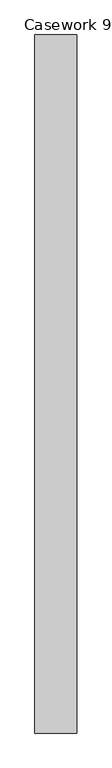
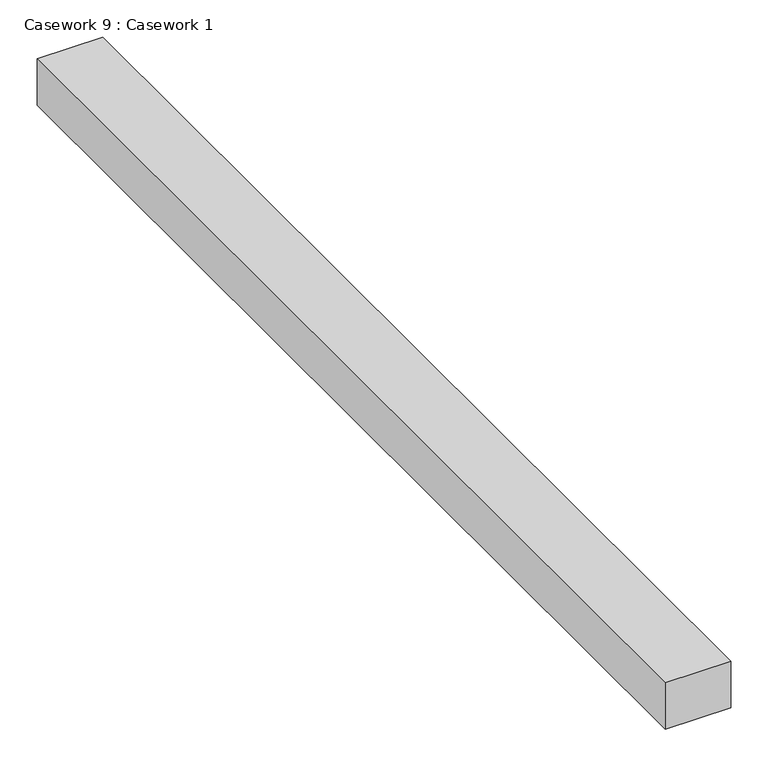
"""IFC4 building model written with IfcOpenShell, lengths in millimetres: furniture geometry, Casework 9 : Casework 1."""

from ifc_helpers import new_model, si_unit, frame, origin, place, context, project, spatial, polyline, outline, extrude, source, transform, mapped, element, save


def casework_9_casework_1_7a666160(model_context):
    return source(origin(), model_context, "Body", "SweptSolid", [
        extrude(outline(polyline([(7224.1559589, 14787.9496924), (7224.1559589, 13098.8496924), (7122.5559589, 13098.8496924), (7122.5559589, 14787.9496924), (7224.1559589, 14787.9496924)])), frame((0.0, 0.0, 3581.4), z_axis=(0.0, 0.0, 1.0), x_axis=(1.0, 0.0, 0.0)), (0.0, 0.0, 1.0), 76.2),
    ])


if __name__ == "__main__":
    model = new_model("IFC4")
    model_context = context("Model", 3, world=origin())
    ifc_project = project(units=[si_unit("LENGTHUNIT", "METRE", prefix="MILLI")], contexts=[model_context])
    site = spatial("IfcSite", under=ifc_project)
    building = spatial("IfcBuilding", under=site)
    placement = place(None, origin())
    casework_9_casework_1_shape = casework_9_casework_1_7a666160(model_context)
    element("IfcFurniture", 1, ObjectType="Casework 9 : Casework 1", at=placement, inside=building, context=model_context, shape_type="MappedRepresentation", body=[
        mapped(casework_9_casework_1_shape, transform((0.0, 0.0, 0.0), x_axis=(1.0, 0.0, 0.0), y_axis=(0.0, 1.0, 0.0), z_axis=(0.0, 0.0, 1.0))),
    ])
    save(model, "model.ifc")

# Revit data of these elements
# Element 1 (IfcFurniture, "Casework 9 : Casework 1")
#   Materials on its faces: "Clad - White"
# Materials
#   "Clad - White": class "Wood", colour RGB 242 242 238, transparency 0, Cost = 0
